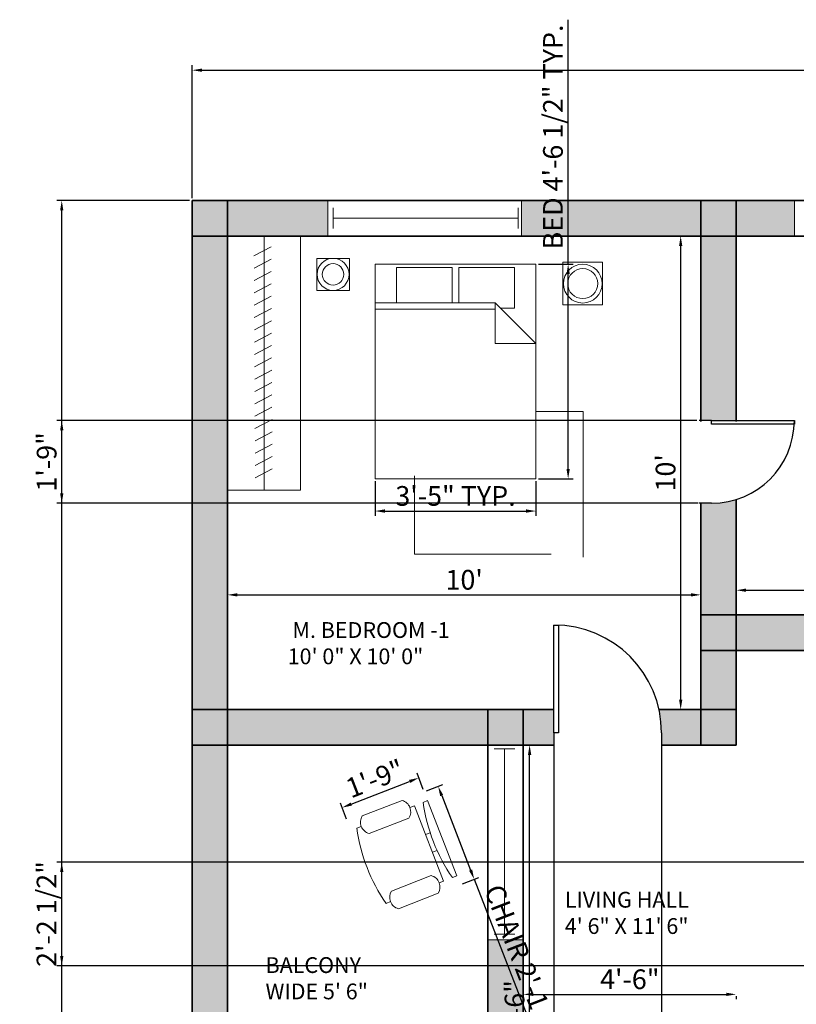
# Model space of a CAD drawing. Units: millimetres. Extents: x 2768 to 4359, y 795 to 1583.
# Tile 3 of 13: x 2768 to 2965, y 1286 to 1535. Entities that reach past the tile are written whole.
import ezdxf

# ---------------------------------------------------------------- set-up
doc = ezdxf.new("R2010")
doc.units = ezdxf.units.MM
for name, color, linetype, lineweight in [('A-ANNO-DIMS', 90, 'Continuous', 18), ('A-AREA-IDEN', 190, 'Continuous', 18), ('A-FLOR-CASE', 50, 'Continuous', 18), ('A-FLOR-CASE-PATT', 50, 'Continuous', 13), ('A-WALL-PATT', 140, 'Continuous', 9), ('doors', 10, 'Continuous', 25), ('furniture', 50, 'Continuous', 18), ('walls', 140, 'Continuous', 35), ('windows', 30, 'Continuous', 18)]:
    doc.layers.add(name, color=color, linetype=linetype, lineweight=lineweight)
doc.styles.get("Standard").update_dxf_attribs({"font": 'arial.ttf'})
doc.dimstyles.new('ISO-25', dxfattribs={"dimtxt": 5, "dimasz": 2.5, "dimexe": 1.25, "dimexo": 0.625, "dimtad": 1, "dimdec": 0, "dimlunit": 3, "dimtxsty": 'Standard', "dimcen": 2.5, "dimadec": 0, "dimazin": 0, "dimtfac": 1, "dimtdec": 0, "dimtmove": 0, "dimatfit": 3, "dimfxl": 1, "dimarcsym": 0})

# ---------------------------------------------------------------- blocks, each defined once
blk = doc.blocks.new('*U2')
for p, q in [((0, 0), (0, -6)), ((40, 0), (40, -6))]:
    blk.add_line(p, q)
blk.add_lwpolyline([(0, 0), (0, 40), (1.75, 40), (1.75, 0)], close=True)
blk.add_arc((0, 0), 40, 0, 90)
blk = doc.blocks.new('*U4')
for p, q in [((0, 4), (0, 0)), ((36, 4), (36, 0)), ((0, 2), (36, 2))]:
    blk.add_line(p, q)
blk = doc.blocks.new('Bed - Queen')
for p, q in [((0, -80.00003), (0, 0)), ((0, 0), (59.99999, 0)), ((59.99999, 0), (59.99999, -80.00003)), ((7.99999, -1.2), (28.79998, -1.2)), ((7.99999, -14.4), (7.99999, -1.2)), ((28.79998, -1.2), (28.79998, -14.4)), ((31.19999, -1.2), (51.99999, -1.2)), ((31.19999, -14.4), (31.19999, -1.2)), ((51.99999, -1.2), (51.99999, -16.4)), ((0, -14.4), (44.8, -14.4)), ((59.99999, -29.6), (44.8, -14.4)), ((44.8, -14.4), (44.8, -29.6)), ((44.8, -16.8), (0, -16.8)), ((51.99999, -16.4), (46.79936, -16.4)), ((44.8, -29.6), (59.99999, -29.6)), ((59.99999, -80.00003), (0, -80.00003))]:
    blk.add_line(p, q)
blk = doc.blocks.new('Chair - Desk')
for p, q in [((-8.5, 0), (-8.5, -1)), ((-8.5, 0), (8.5, 0)), ((8.5, 0), (8.5, -1)), ((-2, -3), (-2, -1.9355)), ((2, -1.9576), (2, -3)), ((-8.5, -3), (-8.5, -4)), ((-8.5, -3), (8.5, -3)), ((8.5, -3), (8.5, -4)), ((-10.5, -5), (-10.5, -14)), ((-6.5, -14), (-6.5, -5)), ((6.5, -5), (6.5, -14)), ((10.5, -14), (10.5, -5)), ((-8.5, -15), (-8.5, -16)), ((8.5, -15), (8.5, -16))]:
    blk.add_line(p, q)
for centre, radius, start, end in [((0, 34.625), 36.625, 256.5803, 283.4197), ((-8.5, -6.5), 2.5, 36.8699, 143.1301), ((8.5, -6.5), 2.5, 36.8699, 143.1301), ((-8.5, -12.5), 2.5, 216.8699, 323.1301), ((8.5, -12.5), 2.5, 216.8699, 323.1301), ((0, 19.625), 36.625, 256.5803, 283.4197)]:
    blk.add_arc(centre, radius, start, end)
blk = doc.blocks.new('*D13')
at = {"layer": 'A-ANNO-DIMS', "color": 0, "lineweight": -2, "transparency": 16777216}
for p, q in [((2934.98, 1480.41), (2934.06, 1480.41)), ((2935.31, 1477.91), (2935.31, 1362.91)), ((2934.98, 1360.41), (2934.06, 1360.41))]:
    blk.add_line(p, q, dxfattribs=at)
at = {"layer": 'A-ANNO-DIMS', "color": 0, "transparency": 16777216}
for points in [[(2934.9, 1477.91), (2935.73, 1477.91), (2935.31, 1480.41)], [(2934.9, 1362.91), (2935.73, 1362.91), (2935.31, 1360.41)]]:
    blk.add_solid(points, dxfattribs=at)
at = {"layer": 'Defpoints', "color": 0, "transparency": 16777216}
for p in [(2935.61, 1480.41), (2935.31, 1360.41), (2935.61, 1360.41)]:
    blk.add_point(p, dxfattribs=at)
at = {"layer": 'A-ANNO-DIMS', "color": 0, "transparency": 16777216, "insert": (2932.13, 1420.41), "char_height": 5, "attachment_point": 5, "rotation": 90}
blk.add_mtext("10'", dxfattribs=at)
blk = doc.blocks.new('*D14')
at = {"layer": 'A-ANNO-DIMS', "color": 0, "lineweight": -2, "transparency": 16777216}
for p, q in [((2820.41, 1390.09), (2820.41, 1390.72)), ((2940.41, 1390.09), (2940.41, 1390.72)), ((2822.91, 1389.47), (2937.91, 1389.47))]:
    blk.add_line(p, q, dxfattribs=at)
at = {"layer": 'A-ANNO-DIMS', "color": 0, "transparency": 16777216}
for points in [[(2822.91, 1389.89), (2822.91, 1389.05), (2820.41, 1389.47)], [(2937.91, 1389.89), (2937.91, 1389.05), (2940.41, 1389.47)]]:
    blk.add_solid(points, dxfattribs=at)
at = {"layer": 'Defpoints', "color": 0, "transparency": 16777216}
for p in [(2820.41, 1389.47), (2940.41, 1389.47), (2940.41, 1389.47)]:
    blk.add_point(p, dxfattribs=at)
at = {"layer": 'A-ANNO-DIMS', "color": 0, "transparency": 16777216, "insert": (2880.41, 1392.65), "char_height": 5, "attachment_point": 5}
blk.add_mtext("10'", dxfattribs=at)
blk = doc.blocks.new('*D16')
at = {"layer": 'A-ANNO-DIMS', "color": 0, "lineweight": -2, "transparency": 16777216}
for p, q in [((2949.41, 1391.28), (2949.41, 1391.9)), ((2951.91, 1390.65), (3006.91, 1390.65)), ((3009.41, 1391.28), (3009.41, 1391.9))]:
    blk.add_line(p, q, dxfattribs=at)
at = {"layer": 'A-ANNO-DIMS', "color": 0, "transparency": 16777216}
for points in [[(2951.91, 1391.07), (2951.91, 1390.23), (2949.41, 1390.65)], [(3006.91, 1391.07), (3006.91, 1390.23), (3009.41, 1390.65)]]:
    blk.add_solid(points, dxfattribs=at)
at = {"layer": 'Defpoints', "color": 0, "transparency": 16777216}
for p in [(2949.41, 1390.65), (3009.41, 1390.65), (3009.41, 1390.65)]:
    blk.add_point(p, dxfattribs=at)
at = {"layer": 'A-ANNO-DIMS', "color": 0, "transparency": 16777216, "insert": (2979.41, 1393.82), "char_height": 5, "attachment_point": 5}
blk.add_mtext("5'", dxfattribs=at)
blk = doc.blocks.new('*D31')
at = {"layer": 'A-ANNO-DIMS', "color": 0, "lineweight": -2, "transparency": 16777216}
for p, q in [((2897.64, 1351.41), (2898.26, 1351.41)), ((2897.01, 1215.91), (2897.01, 1348.91)), ((2897.72, 1213.41), (2895.76, 1213.41))]:
    blk.add_line(p, q, dxfattribs=at)
at = {"layer": 'A-ANNO-DIMS', "color": 0, "transparency": 16777216}
for points in [[(2896.59, 1348.91), (2897.43, 1348.91), (2897.01, 1351.41)], [(2896.59, 1215.91), (2897.43, 1215.91), (2897.01, 1213.41)]]:
    blk.add_solid(points, dxfattribs=at)
at = {"layer": 'Defpoints', "color": 0, "transparency": 16777216}
for p in [(2897.01, 1351.41), (2897.01, 1351.41), (2898.34, 1213.41)]:
    blk.add_point(p, dxfattribs=at)
at = {"layer": 'A-ANNO-DIMS', "color": 0, "transparency": 16777216, "insert": (2893.83, 1282.41), "char_height": 5, "attachment_point": 5, "rotation": 90}
blk.add_mtext('11\'-6"', dxfattribs=at)
blk = doc.blocks.new('*D32')
at = {"layer": 'A-ANNO-DIMS', "color": 0, "lineweight": -2, "transparency": 16777216}
for p, q in [((2897.91, 1288.21), (2946.91, 1288.21)), ((2949.41, 1287.78), (2949.41, 1286.96)), ((2895.41, 1287.64), (2895.41, 1286.96))]:
    blk.add_line(p, q, dxfattribs=at)
at = {"layer": 'A-ANNO-DIMS', "color": 0, "transparency": 16777216}
for points in [[(2897.91, 1288.63), (2897.91, 1287.8), (2895.41, 1288.21)], [(2946.91, 1288.63), (2946.91, 1287.8), (2949.41, 1288.21)]]:
    blk.add_solid(points, dxfattribs=at)
at = {"layer": 'Defpoints', "color": 0, "transparency": 16777216}
for p in [(2895.41, 1288.26), (2949.41, 1288.41), (2949.41, 1288.21)]:
    blk.add_point(p, dxfattribs=at)
at = {"layer": 'A-ANNO-DIMS', "color": 0, "transparency": 16777216, "insert": (2922.41, 1291.39), "char_height": 5, "attachment_point": 5}
blk.add_mtext('4\'-6"', dxfattribs=at)
blk = doc.blocks.new('*D83')
at = {"layer": 'A-ANNO-DIMS', "color": 0, "lineweight": -2, "transparency": 16777216}
for p, q in [((2870.86, 1339.78), (2874.98, 1341.38)), ((2874.71, 1338.6), (2882.05, 1319.7)), ((2880, 1316.23), (2884.12, 1317.83)), ((2882.95, 1317.37), (2901.88, 1268.61))]:
    blk.add_line(p, q, dxfattribs=at)
at = {"layer": 'A-ANNO-DIMS', "color": 0, "transparency": 16777216}
for points in [[(2875.1, 1338.75), (2874.33, 1338.45), (2873.81, 1340.93)], [(2882.44, 1319.85), (2881.66, 1319.55), (2882.95, 1317.37)]]:
    blk.add_solid(points, dxfattribs=at)
at = {"layer": 'Defpoints', "color": 0, "transparency": 16777216}
for p in [(2870.28, 1339.56), (2879.42, 1316), (2882.95, 1317.37)]:
    blk.add_point(p, dxfattribs=at)
at = {"layer": 'A-ANNO-DIMS', "color": 0, "transparency": 16777216, "insert": (2895.86, 1292.99), "char_height": 5, "attachment_point": 5, "rotation": 291.2165}
blk.add_mtext('CHAIR 2\'-1 1/2"', dxfattribs=at)
blk = doc.blocks.new('*D84')
at = {"layer": 'A-ANNO-DIMS', "color": 0, "lineweight": -2, "transparency": 16777216}
for p, q in [((2870.05, 1340.14), (2868.45, 1344.26)), ((2851.79, 1336.45), (2866.57, 1342.19)), ((2850.61, 1332.59), (2849.01, 1336.71))]:
    blk.add_line(p, q, dxfattribs=at)
at = {"layer": 'A-ANNO-DIMS', "color": 0, "transparency": 16777216}
for points in [[(2866.42, 1342.57), (2866.73, 1341.8), (2868.9, 1343.09)], [(2851.64, 1336.84), (2851.94, 1336.06), (2849.46, 1335.54)]]:
    blk.add_solid(points, dxfattribs=at)
at = {"layer": 'Defpoints', "color": 0, "transparency": 16777216}
for p in [(2868.9, 1343.09), (2870.28, 1339.56), (2850.83, 1332.01)]:
    blk.add_point(p, dxfattribs=at)
at = {"layer": 'A-ANNO-DIMS', "color": 0, "transparency": 16777216, "insert": (2858.03, 1342.28), "char_height": 5, "attachment_point": 5, "rotation": 21.2165}
blk.add_mtext('1\'-9"', dxfattribs=at)
blk = doc.blocks.new('*D95')
at = {"layer": 'A-ANNO-DIMS', "color": 0, "lineweight": -2, "transparency": 16777216}
for p, q in [((2906.78, 1473.3), (2906.78, 1535.26)), ((2899.24, 1473.3), (2908.03, 1473.3)), ((2906.78, 1421.38), (2906.78, 1470.8)), ((2899.24, 1418.88), (2908.03, 1418.88))]:
    blk.add_line(p, q, dxfattribs=at)
at = {"layer": 'A-ANNO-DIMS', "color": 0, "transparency": 16777216}
for points in [[(2906.36, 1470.8), (2907.19, 1470.8), (2906.78, 1473.3)], [(2906.36, 1421.38), (2907.19, 1421.38), (2906.78, 1418.88)]]:
    blk.add_solid(points, dxfattribs=at)
at = {"layer": 'Defpoints', "color": 0, "transparency": 16777216}
for p in [(2898.62, 1473.3), (2906.78, 1473.3), (2898.62, 1418.88)]:
    blk.add_point(p, dxfattribs=at)
at = {"layer": 'A-ANNO-DIMS', "color": 0, "transparency": 16777216, "insert": (2903.57, 1505.53), "char_height": 5, "attachment_point": 5, "rotation": 90}
blk.add_mtext('BED 4\'-6 1/2" TYP.', dxfattribs=at)
blk = doc.blocks.new('*D96')
at = {"layer": 'A-ANNO-DIMS', "color": 0, "lineweight": -2, "transparency": 16777216}
for p, q in [((2857.8, 1418.26), (2857.8, 1409.47)), ((2898.62, 1418.26), (2898.62, 1409.47)), ((2860.3, 1410.72), (2896.12, 1410.72))]:
    blk.add_line(p, q, dxfattribs=at)
at = {"layer": 'A-ANNO-DIMS', "color": 0, "transparency": 16777216}
for points in [[(2860.3, 1411.14), (2860.3, 1410.3), (2857.8, 1410.72)], [(2896.12, 1411.14), (2896.12, 1410.3), (2898.62, 1410.72)]]:
    blk.add_solid(points, dxfattribs=at)
at = {"layer": 'Defpoints', "color": 0, "transparency": 16777216}
for p in [(2857.8, 1418.88), (2898.62, 1418.88), (2898.62, 1410.72)]:
    blk.add_point(p, dxfattribs=at)
at = {"layer": 'A-ANNO-DIMS', "color": 0, "transparency": 16777216, "insert": (2878.21, 1413.9), "char_height": 5, "attachment_point": 5}
blk.add_mtext('3\'-5" TYP.', dxfattribs=at)
blk = doc.blocks.new('*D125')
at = {"layer": 'A-ANNO-DIMS', "color": 0, "lineweight": -2, "transparency": 16777216}
for p, q in [((2811.41, 1490.03), (2811.41, 1523.71)), ((2813.91, 1522.46), (3464.91, 1522.46)), ((3467.41, 1490.03), (3467.41, 1523.71))]:
    blk.add_line(p, q, dxfattribs=at)
at = {"layer": 'A-ANNO-DIMS', "color": 0, "transparency": 16777216}
for points in [[(2813.91, 1522.87), (2813.91, 1522.04), (2811.41, 1522.46)], [(3464.91, 1522.87), (3464.91, 1522.04), (3467.41, 1522.46)]]:
    blk.add_solid(points, dxfattribs=at)
at = {"layer": 'Defpoints', "color": 0, "transparency": 16777216}
for p in [(3467.41, 1522.46), (2811.41, 1489.41), (3467.41, 1489.41)]:
    blk.add_point(p, dxfattribs=at)
at = {"layer": 'A-ANNO-DIMS', "color": 0, "transparency": 16777216, "insert": (3139.41, 1525.63), "char_height": 5, "attachment_point": 5}
blk.add_mtext('54\'-8"', dxfattribs=at)
blk = doc.blocks.new('*D127')
at = {"layer": 'A-ANNO-DIMS', "color": 0, "lineweight": -2, "transparency": 16777216}
for p, q in [((2810.78, 1489.41), (2777.11, 1489.41)), ((2778.36, 1013.91), (2778.36, 1486.91)), ((2810.78, 1011.41), (2777.11, 1011.41))]:
    blk.add_line(p, q, dxfattribs=at)
at = {"layer": 'A-ANNO-DIMS', "color": 0, "transparency": 16777216}
for points in [[(2777.94, 1486.91), (2778.77, 1486.91), (2778.36, 1489.41)], [(2777.94, 1013.91), (2778.77, 1013.91), (2778.36, 1011.41)]]:
    blk.add_solid(points, dxfattribs=at)
at = {"layer": 'Defpoints', "color": 0, "transparency": 16777216}
for p in [(2778.36, 1489.41), (2811.41, 1489.41), (2811.41, 1011.41)]:
    blk.add_point(p, dxfattribs=at)
at = {"layer": 'A-ANNO-DIMS', "color": 0, "transparency": 16777216, "insert": (2775.18, 1250.41), "char_height": 5, "attachment_point": 5, "rotation": 90}
blk.add_mtext('39\'-10"', dxfattribs=at)
blk = doc.blocks.new('*D131')
at = {"layer": 'A-ANNO-DIMS', "color": 0, "lineweight": -2, "transparency": 16777216}
for p, q in [((3206.78, 1321.72), (2777.11, 1321.72)), ((2778.36, 1297.93), (2778.36, 1319.22)), ((3206.78, 1295.43), (2777.11, 1295.43))]:
    blk.add_line(p, q, dxfattribs=at)
at = {"layer": 'A-ANNO-DIMS', "color": 0, "transparency": 16777216}
for points in [[(2777.94, 1319.22), (2778.77, 1319.22), (2778.36, 1321.72)], [(2777.94, 1297.93), (2778.77, 1297.93), (2778.36, 1295.43)]]:
    blk.add_solid(points, dxfattribs=at)
at = {"layer": 'Defpoints', "color": 0, "transparency": 16777216}
for p in [(2778.36, 1321.72), (3207.41, 1321.72), (3207.41, 1295.43)]:
    blk.add_point(p, dxfattribs=at)
at = {"layer": 'A-ANNO-DIMS', "color": 0, "transparency": 16777216, "insert": (2775.15, 1308.58), "char_height": 5, "attachment_point": 5, "rotation": 90}
blk.add_mtext('2\'-2 1/2"', dxfattribs=at)
blk = doc.blocks.new('*D133')
at = {"layer": 'A-ANNO-DIMS', "color": 0, "lineweight": -2, "transparency": 16777216}
for p, q in [((2903.16, 1350.78), (2903.16, 856.79)), ((2930.46, 1350.78), (2930.46, 856.79)), ((2905.66, 858.04), (2927.96, 858.04))]:
    blk.add_line(p, q, dxfattribs=at)
at = {"layer": 'A-ANNO-DIMS', "color": 0, "transparency": 16777216}
for points in [[(2905.66, 858.46), (2905.66, 857.63), (2903.16, 858.04)], [(2927.96, 858.46), (2927.96, 857.63), (2930.46, 858.04)]]:
    blk.add_solid(points, dxfattribs=at)
at = {"layer": 'Defpoints', "color": 0, "transparency": 16777216}
for p in [(2903.16, 1351.41), (2930.46, 1351.41), (2930.46, 858.04)]:
    blk.add_point(p, dxfattribs=at)
at = {"layer": 'A-ANNO-DIMS', "color": 0, "transparency": 16777216, "insert": (2916.81, 861.25), "char_height": 5, "attachment_point": 5}
blk.add_mtext('2\'-3 1/2"', dxfattribs=at)
blk = doc.blocks.new('*D134')
at = {"layer": 'A-ANNO-DIMS', "color": 0, "lineweight": -2, "transparency": 16777216}
for p, q in [((2939.38, 1433.68), (2777.11, 1433.68)), ((2778.36, 1415.19), (2778.36, 1431.18)), ((2939.78, 1412.69), (2777.11, 1412.69))]:
    blk.add_line(p, q, dxfattribs=at)
at = {"layer": 'A-ANNO-DIMS', "color": 0, "transparency": 16777216}
for points in [[(2777.94, 1431.18), (2778.77, 1431.18), (2778.36, 1433.68)], [(2777.94, 1415.19), (2778.77, 1415.19), (2778.36, 1412.69)]]:
    blk.add_solid(points, dxfattribs=at)
at = {"layer": 'Defpoints', "color": 0, "transparency": 16777216}
for p in [(2778.36, 1433.68), (2940, 1433.68), (2940.41, 1412.69)]:
    blk.add_point(p, dxfattribs=at)
at = {"layer": 'A-ANNO-DIMS', "color": 0, "transparency": 16777216, "insert": (2775.18, 1423.18), "char_height": 5, "attachment_point": 5, "rotation": 90}
blk.add_mtext('1\'-9"', dxfattribs=at)

msp = doc.modelspace()

# ---------------------------------------------------------------- hatches: boundary and pattern name
at = {"layer": 'A-FLOR-CASE-PATT'}
h = msp.add_hatch(dxfattribs=at)
h.set_pattern_fill('ANSI31', color=256, scale=0.871951, angle=-16.993, style=0)
h.paths.add_polyline_path([(2831.77, 1419.4), (2827.45, 1417.1), (2827.09, 1476.49), (2831.42, 1478.79)])
at = {"layer": 'A-WALL-PATT'}
h = msp.add_hatch(color=256, dxfattribs=at)
h.dxf.hatch_style = 1
h.paths.add_polyline_path([(2820.41, 1480.41), (2811.41, 1480.41), (2811.41, 1360.41), (2820.41, 1360.41)])
h.paths.add_polyline_path([(2820.41, 1489.41), (2811.41, 1489.41), (2811.41, 1480.41), (2820.41, 1480.41)])
h.paths.add_polyline_path([(2845.83, 1489.41), (2820.41, 1489.41), (2820.41, 1480.41), (2845.83, 1480.41)])
h.paths.add_polyline_path([(2940.41, 1489.41), (2894.95, 1489.41), (2894.95, 1480.41), (2940.41, 1480.41)])
h.paths.add_polyline_path([(2949.41, 1489.41), (2940.41, 1489.41), (2940.41, 1480.41), (2949.41, 1480.41)])
h.paths.add_polyline_path([(2949.41, 1480.41), (2940.41, 1480.41), (2940.41, 1433.68), (2943.15, 1433.68), (2949.41, 1433.68)])
h.paths.add_polyline_path([(2964.2, 1489.41), (2949.41, 1489.41), (2949.41, 1480.41), (2964.2, 1480.41)])
h.paths.add_polyline_path([(3018.41, 1489.41), (3009.41, 1489.41), (3009.41, 1480.41), (3018.41, 1480.41)])
h.paths.add_polyline_path([(3009.41, 1489.41), (2990.92, 1489.41), (2990.92, 1480.41), (3009.41, 1480.41)])
h.paths.add_polyline_path([(3018.41, 1480.41), (3009.41, 1480.41), (3009.41, 1384.41), (3018.41, 1384.41)])
h.paths.add_polyline_path([(3009.41, 1384.41), (2949.41, 1384.41), (2949.41, 1375.41), (3009.41, 1375.41)])
h.paths.add_polyline_path([(3018.41, 1384.41), (3009.41, 1384.41), (3009.41, 1375.41), (3018.41, 1375.41)])
h.paths.add_polyline_path([(2949.41, 1384.41), (2940.41, 1384.41), (2940.41, 1375.41), (2949.41, 1375.41)])
h.paths.add_polyline_path([(2949.41, 1413.64, -0.075856), (2943.15, 1412.69), (2940.41, 1412.69), (2940.41, 1384.41), (2949.41, 1384.41)])
h.paths.add_polyline_path([(2949.41, 1375.41), (2940.41, 1375.41), (2940.41, 1360.41), (2949.41, 1360.41)])
h.paths.add_polyline_path([(2949.41, 1360.41), (2940.41, 1360.41), (2940.41, 1351.41), (2949.41, 1351.41)])
h.paths.add_polyline_path([(2940.41, 1360.41), (2929.82, 1360.41, -0.054277), (2930.46, 1354.53), (2930.46, 1351.41), (2940.41, 1351.41)])
h.paths.add_polyline_path([(2903.16, 1354.53), (2903.16, 1360.41), (2895.41, 1360.41), (2895.41, 1351.41), (2903.16, 1351.41)])
h.paths.add_polyline_path([(2886.41, 1360.41), (2820.41, 1360.41), (2820.41, 1351.41), (2886.41, 1351.41)])
h.paths.add_polyline_path([(2895.41, 1360.41), (2886.41, 1360.41), (2886.41, 1351.41), (2895.41, 1351.41)])
h.paths.add_polyline_path([(2820.41, 1360.41), (2811.41, 1360.41), (2811.41, 1351.41), (2820.41, 1351.41)])
h.paths.add_polyline_path([(2820.41, 1351.41), (2811.41, 1351.41), (2811.41, 1213.41), (2820.41, 1213.41)])
h.paths.add_polyline_path([(2886.41, 1213.41), (2820.41, 1213.41), (2820.41, 1204.41), (2886.41, 1204.41)])
h.paths.add_polyline_path([(2820.41, 1213.41), (2811.41, 1213.41), (2811.41, 1204.41), (2820.41, 1204.41)])
h.paths.add_polyline_path([(2895.41, 1302), (2886.41, 1302), (2886.41, 1264.47), (2895.41, 1264.47)])
h.paths.add_polyline_path([(2934.05, 1209.82), (2934.05, 1213.41), (2895.41, 1213.41), (2895.41, 1204.41), (2934.59, 1204.41, -0.049949)])
h.paths.add_polyline_path([(2895.41, 1213.41), (2886.41, 1213.41), (2886.41, 1204.41), (2895.41, 1204.41)])
h.paths.add_polyline_path([(3078.41, 1384.41), (3018.41, 1384.41), (3018.41, 1375.41), (3078.41, 1375.41)])
h.paths.add_polyline_path([(3087.41, 1433.68), (3084.62, 1433.68), (3078.41, 1433.68), (3078.41, 1384.41), (3087.41, 1384.41)])
h.paths.add_polyline_path([(3087.41, 1384.41), (3078.41, 1384.41), (3078.41, 1375.41), (3087.41, 1375.41)])
h.paths.add_polyline_path([(3087.41, 1375.41), (3078.41, 1375.41), (3078.41, 1360.41), (3087.41, 1360.41)])
h.paths.add_polyline_path([(3087.41, 1360.41), (3078.41, 1360.41), (3078.41, 1351.41), (3087.41, 1351.41)])
h.paths.add_polyline_path([(3093.5, 1360.41), (3087.41, 1360.41), (3087.41, 1351.41), (3093.5, 1351.41), (3093.5, 1353.18)])
h.paths.add_polyline_path([(3207.41, 1360.41), (3119.82, 1360.41, -0.067042), (3120.8, 1353.18), (3120.8, 1351.41), (3207.41, 1351.41)])
h.paths.add_polyline_path([(3216.41, 1480.41), (3207.41, 1480.41), (3207.41, 1360.41), (3216.41, 1360.41)])
h.paths.add_polyline_path([(3216.41, 1360.41), (3207.41, 1360.41), (3207.41, 1351.41), (3216.41, 1351.41)])
h.paths.add_polyline_path([(3216.41, 1489.41), (3207.41, 1489.41), (3207.41, 1480.41), (3216.41, 1480.41)])
h.paths.add_polyline_path([(3207.41, 1489.41), (3167.11, 1489.41), (3167.11, 1480.41), (3207.41, 1480.41)])
h.paths.add_polyline_path([(3118.27, 1489.41), (3087.41, 1489.41), (3087.41, 1480.41), (3118.27, 1480.41)])
h.paths.add_polyline_path([(3087.41, 1489.41), (3078.41, 1489.41), (3078.41, 1480.41), (3087.41, 1480.41)])
h.paths.add_polyline_path([(3087.41, 1480.41), (3078.41, 1480.41), (3078.41, 1453.72, -0.07525), (3084.62, 1454.66), (3087.41, 1454.66)])
h.paths.add_polyline_path([(3078.41, 1489.41), (3058.65, 1489.41), (3058.65, 1480.41), (3078.41, 1480.41)])
h.paths.add_polyline_path([(3031.86, 1489.41), (3018.41, 1489.41), (3018.41, 1480.41), (3031.86, 1480.41)])
h.paths.add_polyline_path([(3458.41, 1489.41), (3216.41, 1489.41), (3216.41, 1480.41), (3458.41, 1480.41)])
h.paths.add_polyline_path([(3467.41, 1489.41), (3458.41, 1489.41), (3458.41, 1480.41), (3467.41, 1480.41)])
h.paths.add_polyline_path([(3467.41, 1480.41), (3458.41, 1480.41), (3458.41, 1020.41), (3467.41, 1020.41)])
h.paths.add_polyline_path([(3458.41, 1020.41), (3216.41, 1020.41), (3216.41, 1011.41), (3458.41, 1011.41)])
h.paths.add_polyline_path([(3467.41, 1020.41), (3458.41, 1020.41), (3458.41, 1011.41), (3467.41, 1011.41)])
h.paths.add_polyline_path([(3216.41, 1080.41), (3207.41, 1080.41), (3207.41, 1020.41), (3216.41, 1020.41)])
h.paths.add_polyline_path([(3216.41, 1020.41), (3207.41, 1020.41), (3207.41, 1011.41), (3216.41, 1011.41)])
h.paths.add_polyline_path([(3207.41, 1020.41), (3151.59, 1020.41), (3151.59, 1011.41), (3207.41, 1011.41)])
h.paths.add_polyline_path([(3216.41, 1185.41), (3207.41, 1185.41), (3207.41, 1089.41), (3216.41, 1089.41)])
h.paths.add_polyline_path([(3216.41, 1089.41), (3207.41, 1089.41), (3207.41, 1080.41), (3216.41, 1080.41)])
h.paths.add_polyline_path([(3207.41, 1089.41), (3097.07, 1089.41), (3097.07, 1087.42), (3097.07, 1080.41), (3207.41, 1080.41)])
h.paths.add_polyline_path([(3216.41, 1194.41), (3207.41, 1194.41), (3207.41, 1185.41), (3216.41, 1185.41)])
h.paths.add_polyline_path([(3207.41, 1194.41), (3055.41, 1194.41), (3055.41, 1185.41), (3207.41, 1185.41)])
h.paths.add_polyline_path([(3055.41, 1194.41), (3046.41, 1194.41), (3046.41, 1185.41), (3055.41, 1185.41)])
h.paths.add_polyline_path([(3055.41, 1128.41), (3046.41, 1128.41), (3046.41, 1020.41), (3055.41, 1020.41)])
h.paths.add_polyline_path([(3055.41, 1020.41), (3046.41, 1020.41), (3046.41, 1011.41), (3055.41, 1011.41)])
h.paths.add_polyline_path([(3102.66, 1020.41), (3055.41, 1020.41), (3055.41, 1011.41), (3102.66, 1011.41)])
h.paths.add_polyline_path([(3055.41, 1137.41), (3046.41, 1137.41), (3046.41, 1128.41), (3055.41, 1128.41)])
h.paths.add_polyline_path([(3046.41, 1137.41), (2986.41, 1137.41), (2986.41, 1128.41), (3046.41, 1128.41)])
h.paths.add_polyline_path([(2986.41, 1204.41), (2977.41, 1204.41), (2977.41, 1137.41), (2986.41, 1137.41)])
h.paths.add_polyline_path([(2986.41, 1213.41), (2977.41, 1213.41), (2977.41, 1204.41), (2986.41, 1204.41)])
h.paths.add_polyline_path([(2977.41, 1213.41), (2961.35, 1213.41), (2961.35, 1209.82), (2961.35, 1204.41), (2977.41, 1204.41)])
h.paths.add_polyline_path([(2986.41, 1137.41), (2977.41, 1137.41), (2977.41, 1128.41), (2986.41, 1128.41)])
h.paths.add_polyline_path([(2986.41, 1128.41), (2977.41, 1128.41), (2977.41, 1073.04), (2980.14, 1073.04), (2986.41, 1073.04)])
h.paths.add_polyline_path([(2986.41, 1053, -0.075909), (2980.14, 1052.05), (2977.41, 1052.05), (2977.41, 1020.41), (2986.41, 1020.41)])
h.paths.add_polyline_path([(2986.41, 1020.41), (2977.41, 1020.41), (2977.41, 1011.41), (2986.41, 1011.41)])
h.paths.add_polyline_path([(2977.41, 1020.41), (2903.99, 1020.41), (2903.99, 1011.41), (2977.41, 1011.41)])
h.paths.add_polyline_path([(2820.41, 1111.04), (2811.41, 1111.04), (2811.41, 1020.41), (2820.41, 1020.41)])
h.paths.add_polyline_path([(2820.41, 1020.41), (2811.41, 1020.41), (2811.41, 1011.41), (2820.41, 1011.41)])
h.paths.add_polyline_path([(2855.32, 1020.41), (2820.41, 1020.41), (2820.41, 1011.41), (2855.32, 1011.41)])
h.paths.add_polyline_path([(2820.41, 1204.41), (2811.41, 1204.41), (2811.41, 1161.45), (2820.41, 1161.45)])
edge = h.paths.add_edge_path()
edge.add_arc((3211.84, 1295.2), 27.3, 86.9636, 99.352)
edge.add_line((3207.41, 1322.13), (3207.41, 1351.41))
edge.add_line((3207.41, 1351.41), (3216.41, 1351.41))
edge.add_line((3216.41, 1351.41), (3216.41, 1322.29))
edge.add_line((3216.41, 1322.29), (3213.29, 1322.46))

# ---------------------------------------------------------------- linework, layer by layer
at = {"layer": 'A-FLOR-CASE'}
msp.add_line((2829.66, 1480.41), (2829.66, 1416.05), dxfattribs=at)
msp.add_lwpolyline([(2820.41, 1480.41), (2838.91, 1480.41), (2838.91, 1416.05), (2820.41, 1416.05)], close=True, dxfattribs=at)
at = {"layer": 'furniture'}
for p, q in [((2898.62, 1435.96), (2910.6, 1435.96)), ((2910.6, 1435.96), (2910.6, 1399.04)), ((2867.81, 1399.78), (2867.81, 1419.62)), ((2902.45, 1399.78), (2867.81, 1399.78))]:
    msp.add_line(p, q, dxfattribs=at)
for points in [[(2843.02, 1474.77), (2851.29, 1474.77), (2851.29, 1466.65), (2843.02, 1466.65)], [(2905.44, 1473.76), (2915.51, 1473.76), (2915.51, 1462.97), (2905.44, 1462.97)]]:
    msp.add_lwpolyline(points, close=True, dxfattribs=at)
for centre, radius in [((2847.16, 1470.71), 4.06), ((2847.16, 1470.71), 2.73), ((2910.48, 1468.36), 4.91), ((2910.48, 1468.36), 3.8)]:
    msp.add_circle(centre, radius, dxfattribs=at)
at = {"layer": 'walls'}
for p, q in [((2811.41, 1489.41), (2811.41, 1011.41)), ((2811.41, 1489.41), (3467.41, 1489.41)), ((2820.41, 1489.41), (2820.41, 1351.41)), ((2940.41, 1489.41), (2940.41, 1433.4)), ((2949.41, 1489.41), (2949.41, 1433.4)), ((2811.41, 1480.41), (3467.41, 1480.41)), ((2940.41, 1412.69), (2940.41, 1351.41)), ((2949.41, 1413.64), (2949.41, 1351.41)), ((2940.41, 1384.41), (3018.41, 1384.41)), ((2940.41, 1384.41), (3087.41, 1384.41)), ((2940.41, 1375.41), (3018.41, 1375.41)), ((2940.41, 1375.41), (3087.41, 1375.41)), ((2811.41, 1360.41), (2903.16, 1360.41)), ((2811.41, 1360.41), (2897.01, 1360.41)), ((2886.41, 1360.41), (2886.41, 1204.41)), ((2895.41, 1360.41), (2895.41, 1204.41)), ((2929.82, 1360.41), (2949.41, 1360.41)), ((2939.86, 1360.41), (2949.41, 1360.41)), ((2811.41, 1351.41), (2897.01, 1351.41)), ((2820.41, 1351.41), (2903.16, 1351.41)), ((2820.41, 1351.41), (2820.41, 1204.41)), ((2930.46, 1351.41), (2949.41, 1351.41)), ((2940.04, 1351.41), (2949.41, 1351.41))]:
    msp.add_line(p, q, dxfattribs=at)
at = {"layer": 'windows'}
for p, q in [((2845.83, 1489.41), (2845.83, 1480.41)), ((2894.95, 1489.41), (2894.95, 1480.41)), ((2964.2, 1489.41), (2964.2, 1480.41)), ((2886.41, 1302), (2895.41, 1302))]:
    msp.add_line(p, q, dxfattribs=at)

# ---------------------------------------------------------------- block references
at = {"layer": 'doors', "xscale": 0.5246855638968122, "yscale": 0.5246855638968122, "zscale": 0.5246855638968122, "rotation": 270}
msp.add_blockref('*U2', (2943.15, 1433.68), dxfattribs=at)
at = {"layer": 'doors', "xscale": 0.6824775533392957, "yscale": 0.6824775533392957, "zscale": 0.6824775533392957}
msp.add_blockref('*U2', (2903.16, 1354.53), dxfattribs=at)
at = {"layer": 'furniture', "xscale": 0.6802112050549222, "yscale": 0.6802112050549222, "zscale": 0.6802112050549222}
msp.add_blockref('Bed - Queen', (2857.8, 1473.3), dxfattribs=at)
at = {"layer": 'furniture', "xscale": 1.203277333586112, "yscale": 1.203277333586112, "zscale": 1.203277333586112, "rotation": 291.216509977657}
msp.add_blockref('Chair - Desk', (2874.85, 1327.78), dxfattribs=at)
at = {"layer": 'windows', "xscale": 1.304585616368386, "yscale": 1.304585616368386, "zscale": 1.304585616368386}
msp.add_blockref('*U4', (2847.16, 1482.36), dxfattribs=at)
at = {"layer": 'windows', "xscale": 1.304585616368386, "yscale": 1.304585616368386, "zscale": 1.304585616368386, "rotation": 90}
msp.add_blockref('*U4', (2893.22, 1303.45), dxfattribs=at)

# ---------------------------------------------------------------- texts
at = {"layer": 'A-AREA-IDEN', "char_height": 4, "attachment_point": 1}
for s, width, insert in [(' M. BEDROOM -1 \\P10\' 0" X 10\' 0"', 44.2276, (2835.65, 1382.56)), ('LIVING HALL\\P4\' 6" X 11\' 6"', 39.045, (2905.93, 1314.2)), ('BALCONY\\PWIDE 5\' 6"', 49.0228, (2830.03, 1297.63))]:
    msp.add_mtext_dynamic_manual_height_columns(s, width=width, gutter_width=12.5, heights=[0], dxfattribs=dict(at, insert=insert))

# ---------------------------------------------------------------- dimensions: what is measured, and where the dimension line sits
at = {"layer": 'A-ANNO-DIMS'}
for base, p1, p2, angle, text, picture, middle in [((2906.78, 1473.3), (2898.62, 1418.88), (2898.62, 1473.3), 90, 'BED <> TYP.', '*D95', (2903.57, 1505.53)), ((2882.95, 1317.37), (2870.28, 1339.56), (2879.42, 1316), 291.2165, 'CHAIR <>', '*D83', (2895.86, 1292.99))]:
    dim = msp.add_linear_dim(base=base, p1=p1, p2=p2, angle=angle, text=text, dimstyle='ISO-25', override={"dimdec": 1, "dimlfac": 1, "dimrnd": 0, "dimzin": 1, "dimdsep": 46, "dimlunit": 4, "dimfrac": 2}, dxfattribs=at)
    dim.commit()
    dim.dimension.update_dxf_attribs({"geometry": picture, "text_midpoint": middle})
for base, p1, p2, override, picture, middle in [((3467.41, 1522.46), (2811.41, 1489.41), (3467.41, 1489.41), {"dimdec": 1, "dimlfac": 1, "dimrnd": 0, "dimzin": 1, "dimdsep": 46, "dimlunit": 4, "dimfrac": 2}, '*D125', (3139.41, 1525.63)), ((2940.41, 1389.47), (2820.41, 1389.47), (2940.41, 1389.47), {"dimclrd": 0, "dimclre": 0, "dimclrt": 0}, '*D14', (2880.41, 1392.65)), ((3009.41, 1390.65), (2949.41, 1390.65), (3009.41, 1390.65), {"dimclrd": 0, "dimclre": 0, "dimclrt": 0}, '*D16', (2979.41, 1393.82)), ((2930.46, 858.04), (2903.16, 1351.41), (2930.46, 1351.41), {"dimdec": 1, "dimlfac": 1, "dimrnd": 0, "dimzin": 1, "dimdsep": 46, "dimlunit": 4, "dimfrac": 2}, '*D133', (2916.81, 861.25)), ((2949.41, 1288.21), (2895.41, 1288.26), (2949.41, 1288.41), {"dimclrd": 0, "dimclre": 0, "dimclrt": 0}, '*D32', (2922.41, 1291.39))]:
    dim = msp.add_linear_dim(base=base, p1=p1, p2=p2, dimstyle='ISO-25', override=override, dxfattribs=at)
    dim.commit()
    dim.dimension.update_dxf_attribs({"geometry": picture, "text_midpoint": middle})
for base, p1, p2, angle, override, picture, middle in [((2778.36, 1489.41), (2811.41, 1011.41), (2811.41, 1489.41), 90, {"dimdec": 1, "dimlfac": 1, "dimrnd": 0, "dimzin": 1, "dimdsep": 46, "dimlunit": 4, "dimfrac": 2}, '*D127', (2775.18, 1250.41)), ((2935.31, 1360.41), (2935.61, 1480.41), (2935.61, 1360.41), 90, {"dimclrd": 0, "dimclre": 0, "dimclrt": 0}, '*D13', (2932.13, 1420.41)), ((2778.36, 1433.68), (2940.41, 1412.69), (2940, 1433.68), 90, {"dimdec": 1, "dimlfac": 1, "dimrnd": 0, "dimzin": 1, "dimdsep": 46, "dimlunit": 4, "dimfrac": 2}, '*D134', (2775.18, 1423.18)), ((2897.01, 1351.41), (2898.34, 1213.41), (2897.01, 1351.41), 90, {"dimclrd": 0, "dimclre": 0, "dimclrt": 0}, '*D31', (2893.83, 1282.41)), ((2868.9, 1343.09), (2850.83, 1332.01), (2870.28, 1339.56), 21.2165, {"dimdec": 1, "dimlfac": 1, "dimrnd": 0, "dimzin": 1, "dimdsep": 46, "dimlunit": 4, "dimfrac": 2}, '*D84', (2858.03, 1342.28)), ((2778.36, 1321.72), (3207.41, 1295.43), (3207.41, 1321.72), 90, {"dimdec": 1, "dimlfac": 1, "dimrnd": 0, "dimzin": 1, "dimdsep": 46, "dimlunit": 4, "dimfrac": 2}, '*D131', (2775.15, 1308.58))]:
    dim = msp.add_linear_dim(base=base, p1=p1, p2=p2, angle=angle, dimstyle='ISO-25', override=override, dxfattribs=at)
    dim.commit()
    dim.dimension.update_dxf_attribs({"geometry": picture, "text_midpoint": middle})
dim = msp.add_linear_dim(base=(2898.62, 1410.72), p1=(2857.8, 1418.88), p2=(2898.62, 1418.88), text='<> TYP.', dimstyle='ISO-25', override={"dimdec": 1, "dimlfac": 1, "dimrnd": 0, "dimzin": 1, "dimdsep": 46, "dimlunit": 4, "dimfrac": 2}, dxfattribs=at)
dim.commit()
dim.dimension.update_dxf_attribs({"geometry": '*D96', "text_midpoint": (2878.21, 1413.9)})

doc.saveas('drawing.dxf')
